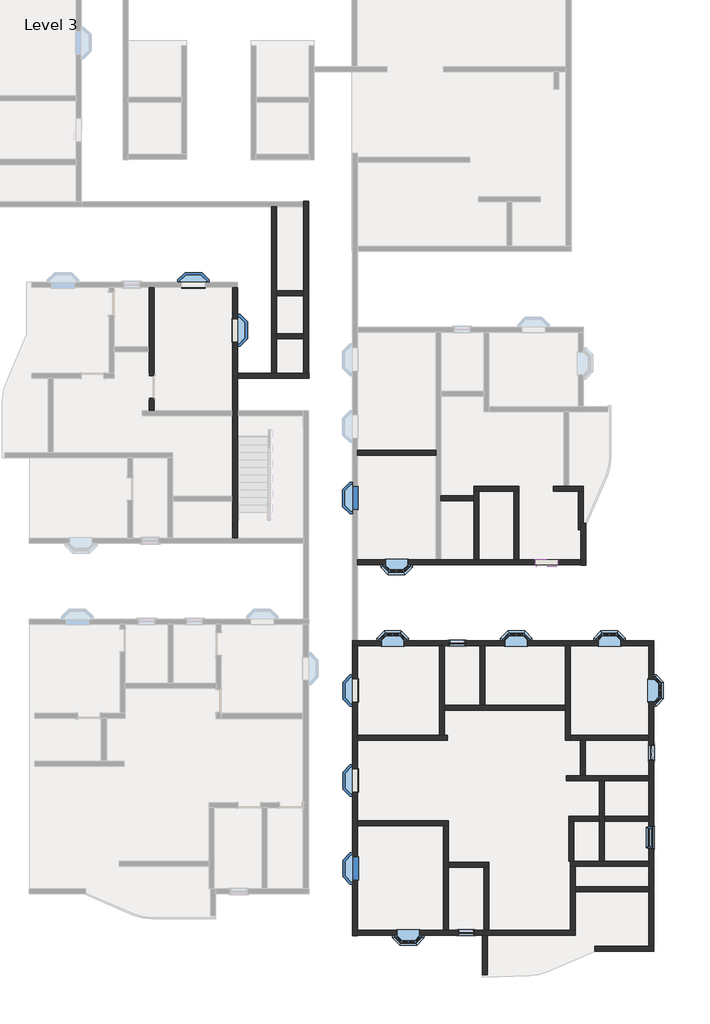
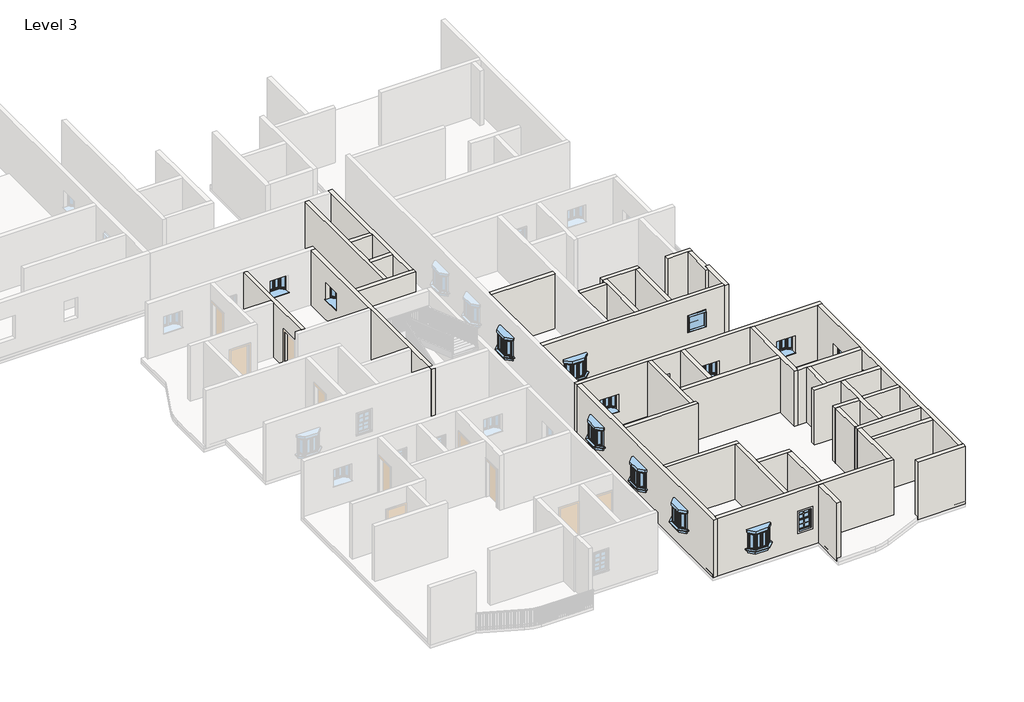
# One storey, part 2 of 14: 40 walls, 17 windows.
"""IFC4 building model written with IfcOpenShell, lengths in millimetres."""

from ifc_helpers import new_model, si_unit, frame, origin, place, context, project, spatial, polyline, outline, extrude, faceted_brep, transform, mapped, element, save
from components import window_910x910mm_67ef725a, window_8debb0fa, windows_sgl_w_glazing_bars_910x910mm_256712d0

model = new_model("IFC4")

# Units and contexts
model_context = context("Model", 3, world=origin())
ifc_project = project(units=[si_unit("LENGTHUNIT", "METRE", prefix="MILLI")], contexts=[model_context])

# Site, building, storey
site = spatial("IfcSite", under=ifc_project)
building = spatial("IfcBuilding", under=site)
storey = spatial("IfcBuildingStorey", under=building, Name="Level 3", Elevation=6096.0)

# Walls
placement = place(None, origin())
element("IfcWall", 1, ObjectType="4.5\" p", at=placement, inside=storey, context=model_context, shape_type="SweptSolid", body=[
    extrude(outline(polyline([(6070.4380523, -28382.7374148), (6070.4380523, -26796.6042694), (6273.6380523, -26796.6042694), (6273.6380523, -28382.7374148), (6070.4380523, -28382.7374148)])), frame((0.0, 0.0, 6096.0), z_axis=(0.0, 0.0, 1.0), x_axis=(1.0, 0.0, 0.0)), (0.0, 0.0, 1.0), 3048.0),
])
element("IfcWall", 2, ObjectType="4.5\" p", at=placement, inside=storey, context=model_context, shape_type="Brep", body=[
    faceted_brep([(10639.6896214, -27431.6042694, 6096.0), (13030.0380523, -27431.6042694, 6096.0), (13030.0380523, -27431.6042694, 9144.0), (10639.6896214, -27431.6042694, 9144.0), (10639.6896214, -27228.4042694, 6096.0), (10639.6896214, -27228.4042694, 9144.0), (12814.1380523, -27228.4042694, 9144.0), (13017.3380523, -27228.4042694, 9144.0), (13030.0380523, -27228.4042694, 9144.0), (13030.0380523, -27228.4042694, 6096.0), (13017.3380523, -27228.4042694, 6096.0), (12814.1380523, -27228.4042694, 6096.0)], [[[0, 1, 2, 3]], [[4, 5, 6, 7, 8, 9, 10, 11]], [[1, 0, 4, 11, 10, 9]], [[2, 1, 9, 8]], [[3, 2, 8, 7, 6, 5]], [[0, 3, 5, 4]]]),
])
element("IfcWall", 3, ObjectType="4.5\" p", at=placement, inside=storey, context=model_context, shape_type="Brep", body=[
    faceted_brep([(1015.8380523, -18878.1542694, 6096.0), (4648.0380523, -18878.1542694, 6096.0), (4648.0380523, -18878.1542694, 9144.0), (1015.8380523, -18878.1542694, 9144.0), (1015.8380523, -18674.9542694, 6096.0), (1015.8380523, -18674.9542694, 9144.0), (4336.8880523, -18674.9542694, 9144.0), (4540.0880523, -18674.9542694, 9144.0), (4648.0380523, -18674.9542694, 9144.0), (4648.0380523, -18674.9542694, 6096.0), (4540.0880523, -18674.9542694, 6096.0), (4336.8880523, -18674.9542694, 6096.0)], [[[0, 1, 2, 3]], [[4, 5, 6, 7, 8, 9, 10, 11]], [[1, 0, 4, 11, 10, 9]], [[2, 1, 9, 8]], [[3, 2, 8, 7, 6, 5]], [[0, 3, 5, 4]]]),
])
element("IfcWall", 4, ObjectType="4.5\" p", at=placement, inside=storey, context=model_context, shape_type="Brep", body=[
    faceted_brep([(4336.8880523, -15049.1042694, 6096.0), (4336.8880523, -18674.9542694, 6096.0), (4336.8880523, -18674.9542694, 9144.0), (4336.8880523, -15049.1042694, 9144.0), (4540.0880523, -15049.1042694, 6096.0), (4540.0880523, -15049.1042694, 9144.0), (4540.0880523, -17455.7542694, 9144.0), (4540.0880523, -17658.9542694, 9144.0), (4540.0880523, -18674.9542694, 9144.0), (4540.0880523, -18674.9542694, 6096.0), (4540.0880523, -17658.9542694, 6096.0), (4540.0880523, -17455.7542694, 6096.0)], [[[0, 1, 2, 3]], [[4, 5, 6, 7, 8, 9, 10, 11]], [[1, 0, 4, 11, 10, 9]], [[3, 2, 8, 7, 6, 5]], [[0, 3, 5, 4]], [[2, 1, 9, 8]]]),
])
element("IfcWall", 5, ObjectType="4.5\" p", at=placement, inside=storey, context=model_context, shape_type="Brep", body=[
    faceted_brep([(4540.0880523, -17658.9542694, 6096.0), (9442.2880523, -17658.9542694, 6096.0), (9442.2880523, -17658.9542694, 9144.0), (4540.0880523, -17658.9542694, 9144.0), (4540.0880523, -17455.7542694, 6096.0), (4540.0880523, -17455.7542694, 9144.0), (5975.1880523, -17455.7542694, 9144.0), (6178.3880523, -17455.7542694, 9144.0), (9442.2880523, -17455.7542694, 9144.0), (9442.2880523, -17455.7542694, 6096.0), (6178.3880523, -17455.7542694, 6096.0), (5975.1880523, -17455.7542694, 6096.0)], [[[0, 1, 2, 3]], [[4, 5, 6, 7, 8, 9, 10, 11]], [[1, 0, 4, 11, 10, 9]], [[3, 2, 8, 7, 6, 5]], [[0, 3, 5, 4]], [[2, 1, 9, 8]]]),
])
element("IfcWall", 6, ObjectType="4.5\" p", at=placement, inside=storey, context=model_context, shape_type="SweptSolid", body=[
    extrude(outline(polyline([(5975.1880523, -17455.7542694), (5975.1880523, -15049.1042694), (6178.3880523, -15049.1042694), (6178.3880523, -17455.7542694), (5975.1880523, -17455.7542694)])), frame((0.0, 0.0, 6096.0), z_axis=(0.0, 0.0, 1.0), x_axis=(1.0, 0.0, 0.0)), (0.0, 0.0, 1.0), 3048.0),
])
element("IfcWall", 7, ObjectType="4.5\" p", at=placement, inside=storey, context=model_context, shape_type="Brep", body=[
    faceted_brep([(9442.2880523, -15049.1042694, 6096.0), (9442.2880523, -17455.7542694, 6096.0), (9442.2880523, -17658.9542694, 6096.0), (9442.2880523, -18871.8042694, 6096.0), (9442.2880523, -18871.8042694, 9144.0), (9442.2880523, -17658.9542694, 9144.0), (9442.2880523, -17455.7542694, 9144.0), (9442.2880523, -15049.1042694, 9144.0), (9645.4880523, -15049.1042694, 6096.0), (9645.4880523, -15049.1042694, 9144.0), (9645.4880523, -18668.6042694, 9144.0), (9645.4880523, -18871.8042694, 9144.0), (9645.4880523, -18871.8042694, 6096.0), (9645.4880523, -18668.6042694, 6096.0)], [[[0, 1, 2, 3, 4, 5, 6, 7]], [[8, 9, 10, 11, 12, 13]], [[3, 2, 1, 0, 8, 13, 12]], [[7, 6, 5, 4, 11, 10, 9]], [[0, 7, 9, 8]], [[4, 3, 12, 11]]]),
])
element("IfcWall", 8, ObjectType="4.5\" p", at=placement, inside=storey, context=model_context, shape_type="Brep", body=[
    faceted_brep([(1015.8380523, -22345.2542694, 6096.0), (4489.2880523, -22345.2542694, 6096.0), (4692.4880523, -22345.2542694, 6096.0), (4692.4880523, -22345.2542694, 9144.0), (4489.2880523, -22345.2542694, 9144.0), (1015.8380523, -22345.2542694, 9144.0), (1015.8380523, -22142.0542694, 6096.0), (1015.8380523, -22142.0542694, 9144.0), (4692.4880523, -22142.0542694, 9144.0), (4692.4880523, -22142.0542694, 6096.0)], [[[0, 1, 2, 3, 4, 5]], [[6, 7, 8, 9]], [[2, 1, 0, 6, 9]], [[5, 4, 3, 8, 7]], [[0, 5, 7, 6]], [[3, 2, 9, 8]]]),
])
element("IfcWall", 9, ObjectType="4.5\" p", at=placement, inside=storey, context=model_context, shape_type="Brep", body=[
    faceted_brep([(4489.2880523, -22345.2542694, 6096.0), (4489.2880523, -26580.7042694, 6096.0), (4489.2880523, -26580.7042694, 9144.0), (4489.2880523, -22345.2542694, 9144.0), (4692.4880523, -22345.2542694, 6096.0), (4692.4880523, -22345.2542694, 9144.0), (4692.4880523, -23818.4542694, 9144.0), (4692.4880523, -24021.6542694, 9144.0), (4692.4880523, -26580.7042694, 9144.0), (4692.4880523, -26580.7042694, 6096.0), (4692.4880523, -24021.6542694, 6096.0), (4692.4880523, -23818.4542694, 6096.0)], [[[0, 1, 2, 3]], [[4, 5, 6, 7, 8, 9, 10, 11]], [[1, 0, 4, 11, 10, 9]], [[3, 2, 8, 7, 6, 5]], [[0, 3, 5, 4]], [[2, 1, 9, 8]]]),
])
element("IfcWall", 10, ObjectType="4.5\" p", at=placement, inside=storey, context=model_context, shape_type="Brep", body=[
    faceted_brep([(4692.4880523, -24021.6542694, 6096.0), (6127.5880523, -24021.6542694, 6096.0), (6330.7880523, -24021.6542694, 6096.0), (6330.7880523, -24021.6542694, 9144.0), (6127.5880523, -24021.6542694, 9144.0), (4692.4880523, -24021.6542694, 9144.0), (4692.4880523, -23818.4542694, 6096.0), (4692.4880523, -23818.4542694, 9144.0), (6330.7880523, -23818.4542694, 9144.0), (6330.7880523, -23818.4542694, 6096.0)], [[[0, 1, 2, 3, 4, 5]], [[6, 7, 8, 9]], [[2, 1, 0, 6, 9]], [[5, 4, 3, 8, 7]], [[0, 5, 7, 6]], [[3, 2, 9, 8]]]),
])
element("IfcWall", 11, ObjectType="4.5\" p", at=placement, inside=storey, context=model_context, shape_type="SweptSolid", body=[
    extrude(outline(polyline([(6127.5880523, -26580.7042694), (6127.5880523, -24021.6542694), (6330.7880523, -24021.6542694), (6330.7880523, -26580.7042694), (6127.5880523, -26580.7042694)])), frame((0.0, 0.0, 6096.0), z_axis=(0.0, 0.0, 1.0), x_axis=(1.0, 0.0, 0.0)), (0.0, 0.0, 1.0), 3048.0),
])
element("IfcWall", 12, ObjectType="4.5\" p", at=placement, inside=storey, context=model_context, shape_type="Brep", body=[
    faceted_brep([(9645.4880523, -18871.8042694, 6096.0), (10051.8880523, -18871.8042694, 6096.0), (10255.0880523, -18871.8042694, 6096.0), (12814.1380523, -18871.8042694, 6096.0), (12814.1380523, -18871.8042694, 9144.0), (10255.0880523, -18871.8042694, 9144.0), (10051.8880523, -18871.8042694, 9144.0), (9645.4880523, -18871.8042694, 9144.0), (9645.4880523, -18668.6042694, 6096.0), (9645.4880523, -18668.6042694, 9144.0), (12814.1380523, -18668.6042694, 9144.0), (12814.1380523, -18668.6042694, 6096.0)], [[[0, 1, 2, 3, 4, 5, 6, 7]], [[8, 9, 10, 11]], [[3, 2, 1, 0, 8, 11]], [[7, 6, 5, 4, 10, 9]], [[0, 7, 9, 8]], [[4, 3, 11, 10]]]),
])
element("IfcWall", 13, ObjectType="4.5\" p", at=placement, inside=storey, context=model_context, shape_type="SweptSolid", body=[
    extrude(outline(polyline([(10051.8880523, -20313.2542694), (10051.8880523, -18871.8042694), (10255.0880523, -18871.8042694), (10255.0880523, -20313.2542694), (10051.8880523, -20313.2542694)])), frame((0.0, 0.0, 6096.0), z_axis=(0.0, 0.0, 1.0), x_axis=(1.0, 0.0, 0.0)), (0.0, 0.0, 1.0), 3048.0),
])
element("IfcWall", 14, ObjectType="4.5\" p", at=placement, inside=storey, context=model_context, shape_type="Brep", body=[
    faceted_brep([(12814.1380523, -20313.2542694, 6096.0), (10255.0880523, -20313.2542694, 6096.0), (10051.8880523, -20313.2542694, 6096.0), (9486.7380523, -20313.2542694, 6096.0), (9486.7380523, -20313.2542694, 9144.0), (10051.8880523, -20313.2542694, 9144.0), (10255.0880523, -20313.2542694, 9144.0), (12814.1380523, -20313.2542694, 9144.0), (12814.1380523, -20516.4542694, 6096.0), (12814.1380523, -20516.4542694, 9144.0), (11017.0880523, -20516.4542694, 9144.0), (10813.8880523, -20516.4542694, 9144.0), (9486.7380523, -20516.4542694, 9144.0), (9486.7380523, -20516.4542694, 6096.0), (10813.8880523, -20516.4542694, 6096.0), (11017.0880523, -20516.4542694, 6096.0)], [[[0, 1, 2, 3, 4, 5, 6, 7]], [[8, 9, 10, 11, 12, 13, 14, 15]], [[3, 2, 1, 0, 8, 15, 14, 13]], [[4, 3, 13, 12]], [[7, 6, 5, 4, 12, 11, 10, 9]], [[0, 7, 9, 8]]]),
])
element("IfcWall", 15, ObjectType="4.5\" p", at=placement, inside=storey, context=model_context, shape_type="Brep", body=[
    faceted_brep([(10813.8880523, -20516.4542694, 6096.0), (10813.8880523, -21951.5542694, 6096.0), (10813.8880523, -22154.7542694, 6096.0), (10813.8880523, -23779.5416506, 6096.0), (10813.8880523, -23779.5416506, 9144.0), (10813.8880523, -22154.7542694, 9144.0), (10813.8880523, -21951.5542694, 9144.0), (10813.8880523, -20516.4542694, 9144.0), (11017.0880523, -20516.4542694, 6096.0), (11017.0880523, -20516.4542694, 9144.0), (11017.0880523, -21951.5542694, 9144.0), (11017.0880523, -22154.7542694, 9144.0), (11017.0880523, -23779.5416506, 9144.0), (11017.0880523, -23779.5416506, 6096.0), (11017.0880523, -22154.7542694, 6096.0), (11017.0880523, -21951.5542694, 6096.0)], [[[0, 1, 2, 3, 4, 5, 6, 7]], [[8, 9, 10, 11, 12, 13, 14, 15]], [[3, 2, 1, 0, 8, 15, 14, 13]], [[7, 6, 5, 4, 12, 11, 10, 9]], [[0, 7, 9, 8]], [[4, 3, 13, 12]]]),
])
element("IfcWall", 16, ObjectType="4.5\" p", at=placement, inside=storey, context=model_context, shape_type="Brep", body=[
    faceted_brep([(12814.1380523, -23779.5416506, 6096.0), (11017.0880523, -23779.5416506, 6096.0), (10813.8880523, -23779.5416506, 6096.0), (9791.5380523, -23779.5416506, 6096.0), (9632.7880523, -23779.5416506, 6096.0), (9632.7880523, -23779.5416506, 9144.0), (9791.5380523, -23779.5416506, 9144.0), (10813.8880523, -23779.5416506, 9144.0), (11017.0880523, -23779.5416506, 9144.0), (12814.1380523, -23779.5416506, 9144.0), (12814.1380523, -23982.7416506, 6096.0), (12814.1380523, -23982.7416506, 9144.0), (9835.9880523, -23982.7416506, 9144.0), (9632.7880523, -23982.7416506, 9144.0), (9632.7880523, -23982.7416506, 6096.0), (9835.9880523, -23982.7416506, 6096.0)], [[[0, 1, 2, 3, 4, 5, 6, 7, 8, 9]], [[10, 11, 12, 13, 14, 15]], [[4, 3, 2, 1, 0, 10, 15, 14]], [[9, 8, 7, 6, 5, 13, 12, 11]], [[0, 9, 11, 10]], [[5, 4, 14, 13]]]),
])
element("IfcWall", 17, ObjectType="4.5\" p", at=placement, inside=storey, context=model_context, shape_type="Brep", body=[
    faceted_brep([(9632.7880523, -23982.7416506, 6096.0), (9632.7880523, -26580.7042694, 6096.0), (9632.7880523, -26580.7042694, 9144.0), (9632.7880523, -23982.7416506, 9144.0), (9835.9880523, -23982.7416506, 6096.0), (9835.9880523, -23982.7416506, 9144.0), (9835.9880523, -24805.3496998, 9144.0), (9835.9880523, -25008.5496998, 9144.0), (9835.9880523, -26580.7042694, 9144.0), (9835.9880523, -26580.7042694, 6096.0), (9835.9880523, -25008.5496998, 6096.0), (9835.9880523, -24805.3496998, 6096.0)], [[[0, 1, 2, 3]], [[4, 5, 6, 7, 8, 9, 10, 11]], [[1, 0, 4, 11, 10, 9]], [[3, 2, 8, 7, 6, 5]], [[2, 1, 9, 8]], [[0, 3, 5, 4]]]),
])
element("IfcWall", 18, ObjectType="4.5\" p", at=placement, inside=storey, context=model_context, shape_type="SweptSolid", body=[
    extrude(outline(polyline([(12814.1380523, -25008.5496998), (9835.9880523, -25008.5496998), (9835.9880523, -24805.3496998), (12814.1380523, -24805.3496998), (12814.1380523, -25008.5496998)])), frame((0.0, 0.0, 6096.0), z_axis=(0.0, 0.0, 1.0), x_axis=(1.0, 0.0, 0.0)), (0.0, 0.0, 1.0), 3048.0),
])
element("IfcWall", 19, ObjectType="4.5\" p", at=placement, inside=storey, context=model_context, shape_type="Brep", body=[
    faceted_brep([(-7432.737215, -5015.2916506, 8229.6), (-7432.737215, -5015.2916506, 6096.0), (-7432.737215, -5523.2916506, 6096.0), (-7432.737215, -5523.2916506, 9144.0), (-7432.737215, -3135.6916506, 9144.0), (-7432.737215, -2932.4916506, 9144.0), (-7432.737215, -525.8416506, 9144.0), (-7432.737215, -525.8416506, 6096.0), (-7432.737215, -2932.4916506, 6096.0), (-7432.737215, -3135.6916506, 6096.0), (-7432.737215, -4100.8916506, 6096.0), (-7432.737215, -4100.8916506, 8229.6), (-7229.537215, -5523.2916506, 6096.0), (-7229.537215, -5015.2916506, 6096.0), (-7229.537215, -5015.2916506, 8229.6), (-7229.537215, -4100.8916506, 8229.6), (-7229.537215, -4100.8916506, 6096.0), (-7229.537215, -525.8416506, 6096.0), (-7229.537215, -525.8416506, 9144.0), (-7229.537215, -5523.2916506, 9144.0)], [[[0, 1, 2, 3, 4, 5, 6, 7, 8, 9, 10, 11]], [[12, 13, 14, 15, 16, 17, 18, 19]], [[2, 1, 13, 12]], [[10, 9, 8, 7, 17, 16]], [[6, 5, 4, 3, 19, 18]], [[7, 6, 18, 17]], [[3, 2, 12, 19]], [[14, 13, 1, 0]], [[15, 14, 0, 11]], [[16, 15, 11, 10]]]),
])
element("IfcWall", 20, ObjectType="4.5\" p", at=placement, inside=storey, context=model_context, shape_type="Brep", body=[
    faceted_brep([(-3857.687215, -4202.4916506, 6096.0), (-961.4891351, -4202.4916506, 6096.0), (-961.4891351, -4202.4916506, 9144.0), (-3857.687215, -4202.4916506, 9144.0), (-3857.687215, -3999.2916506, 6096.0), (-3857.687215, -3999.2916506, 9144.0), (-2472.7891351, -3999.2916506, 9144.0), (-2269.5891351, -3999.2916506, 9144.0), (-1177.3891351, -3999.2916506, 9144.0), (-974.1891351, -3999.2916506, 9144.0), (-961.4891351, -3999.2916506, 9144.0), (-961.4891351, -3999.2916506, 6096.0), (-974.1891351, -3999.2916506, 6096.0), (-1177.3891351, -3999.2916506, 6096.0), (-2269.5891351, -3999.2916506, 6096.0), (-2472.7891351, -3999.2916506, 6096.0)], [[[0, 1, 2, 3]], [[4, 5, 6, 7, 8, 9, 10, 11, 12, 13, 14, 15]], [[1, 0, 4, 15, 14, 13, 12, 11]], [[2, 1, 11, 10]], [[3, 2, 10, 9, 8, 7, 6, 5]], [[0, 3, 5, 4]]]),
])
element("IfcWall", 21, ObjectType="4.5\" p", at=placement, inside=storey, context=model_context, shape_type="SweptSolid", body=[
    extrude(outline(polyline([(-1177.3891351, -868.7416506), (-2269.5891351, -868.7416506), (-2269.5891351, -665.5416506), (-1177.3891351, -665.5416506), (-1177.3891351, -868.7416506)])), frame((0.0, 0.0, 6096.0), z_axis=(0.0, 0.0, 1.0), x_axis=(1.0, 0.0, 0.0)), (0.0, 0.0, 1.0), 3048.0),
])
element("IfcWall", 22, ObjectType="4.5\" p", at=placement, inside=storey, context=model_context, shape_type="SweptSolid", body=[
    extrude(outline(polyline([(-1177.3891351, -2597.8466506), (-2269.5891351, -2597.8466506), (-2269.5891351, -2394.6466506), (-1177.3891351, -2394.6466506), (-1177.3891351, -2597.8466506)])), frame((0.0, 0.0, 6096.0), z_axis=(0.0, 0.0, 1.0), x_axis=(1.0, 0.0, 0.0)), (0.0, 0.0, 1.0), 3048.0),
])
element("IfcWall", 23, ObjectType="4.5\" p", at=placement, inside=storey, context=model_context, shape_type="SweptSolid", body=[
    extrude(outline(polyline([(5721.1880523, -9162.6542694), (4387.6880523, -9162.6542694), (4387.6880523, -8959.4542694), (5721.1880523, -8959.4542694), (5721.1880523, -9162.6542694)])), frame((0.0, 0.0, 6096.0), z_axis=(0.0, 0.0, 1.0), x_axis=(1.0, 0.0, 0.0)), (0.0, 0.0, 1.0), 3048.0),
])
element("IfcWall", 24, ObjectType="4.5\" p", at=placement, inside=storey, context=model_context, shape_type="Brep", body=[
    faceted_brep([(5721.1880523, -8781.6542694, 6096.0), (5924.3880523, -8781.6542694, 6096.0), (7359.4880523, -8781.6542694, 6096.0), (7562.6880523, -8781.6542694, 6096.0), (7562.6880523, -8781.6542694, 9144.0), (7359.4880523, -8781.6542694, 9144.0), (5924.3880523, -8781.6542694, 9144.0), (5721.1880523, -8781.6542694, 9144.0), (5721.1880523, -8578.4542694, 6096.0), (5721.1880523, -8578.4542694, 9144.0), (7562.6880523, -8578.4542694, 9144.0), (7562.6880523, -8578.4542694, 6096.0)], [[[0, 1, 2, 3, 4, 5, 6, 7]], [[8, 9, 10, 11]], [[3, 2, 1, 0, 8, 11]], [[7, 6, 5, 4, 10, 9]], [[0, 7, 9, 8]], [[4, 3, 11, 10]]]),
])
element("IfcWall", 25, ObjectType="4.5\" p", at=placement, inside=storey, context=model_context, shape_type="Brep", body=[
    faceted_brep([(5721.1880523, -8781.6542694, 6096.0), (5721.1880523, -8959.4542694, 6096.0), (5721.1880523, -9162.6542694, 6096.0), (5721.1880523, -11556.6042694, 6096.0), (5721.1880523, -11556.6042694, 9144.0), (5721.1880523, -9162.6542694, 9144.0), (5721.1880523, -8959.4542694, 9144.0), (5721.1880523, -8781.6542694, 9144.0), (5924.3880523, -8781.6542694, 6096.0), (5924.3880523, -8781.6542694, 9144.0), (5924.3880523, -11556.6042694, 9144.0), (5924.3880523, -11556.6042694, 6096.0)], [[[0, 1, 2, 3, 4, 5, 6, 7]], [[8, 9, 10, 11]], [[3, 2, 1, 0, 8, 11]], [[7, 6, 5, 4, 10, 9]], [[0, 7, 9, 8]], [[4, 3, 11, 10]]]),
])
element("IfcWall", 26, ObjectType="4.5\" p", at=placement, inside=storey, context=model_context, shape_type="SweptSolid", body=[
    extrude(outline(polyline([(7359.4880523, -11556.6042694), (7359.4880523, -8781.6542694), (7562.6880523, -8781.6542694), (7562.6880523, -11556.6042694), (7359.4880523, -11556.6042694)])), frame((0.0, 0.0, 6096.0), z_axis=(0.0, 0.0, 1.0), x_axis=(1.0, 0.0, 0.0)), (0.0, 0.0, 1.0), 3048.0),
])
element("IfcWall", 27, ObjectType="4.5\" p", at=placement, inside=storey, context=model_context, shape_type="SweptSolid", body=[
    extrude(outline(polyline([(4184.4880523, -7333.8542694), (1007.0108649, -7333.8542694), (1007.0108649, -7130.6542694), (4184.4880523, -7130.6542694), (4184.4880523, -7333.8542694)])), frame((0.0, 0.0, 6096.0), z_axis=(0.0, 0.0, 1.0), x_axis=(1.0, 0.0, 0.0)), (0.0, 0.0, 1.0), 3048.0),
])
element("IfcWall", 28, ObjectType="4.5\" p", at=placement, inside=storey, context=model_context, shape_type="Brep", body=[
    faceted_brep([(8953.3380523, -8781.6542694, 6096.0), (9956.6380523, -8781.6542694, 6096.0), (10159.8380523, -8781.6542694, 6096.0), (10172.5380523, -8781.6542694, 6096.0), (10172.5380523, -8781.6542694, 9144.0), (10159.8380523, -8781.6542694, 9144.0), (9956.6380523, -8781.6542694, 9144.0), (8953.3380523, -8781.6542694, 9144.0), (8953.3380523, -8578.4542694, 6096.0), (8953.3380523, -8578.4542694, 9144.0), (9371.2322031, -8578.4542694, 9144.0), (9574.4322031, -8578.4542694, 9144.0), (10172.5380523, -8578.4542694, 9144.0), (10172.5380523, -8578.4542694, 6096.0), (9574.4322031, -8578.4542694, 6096.0), (9371.2322031, -8578.4542694, 6096.0)], [[[0, 1, 2, 3, 4, 5, 6, 7]], [[8, 9, 10, 11, 12, 13, 14, 15]], [[3, 2, 1, 0, 8, 15, 14, 13]], [[4, 3, 13, 12]], [[7, 6, 5, 4, 12, 11, 10, 9]], [[0, 7, 9, 8]]]),
])
element("IfcWall", 29, ObjectType="4.5\" p", at=placement, inside=storey, context=model_context, shape_type="SweptSolid", body=[
    extrude(outline(polyline([(9956.6380523, -10352.8912671), (9956.6380523, -8781.6542694), (10159.8380523, -8781.6542694), (10159.8380523, -10352.8912671), (9956.6380523, -10352.8912671)])), frame((0.0, 0.0, 6096.0), z_axis=(0.0, 0.0, 1.0), x_axis=(1.0, 0.0, 0.0)), (0.0, 0.0, 1.0), 3048.0),
])
element("IfcWall", 30, ObjectType="4.5\" p", at=placement, inside=storey, context=model_context, shape_type="Brep", body=[
    faceted_brep([(12814.1380523, -21951.5542694, 9144.0), (12814.1380523, -21951.5542694, 6096.0), (11017.0880523, -21951.5542694, 6096.0), (11017.0880523, -21951.5542694, 9144.0), (12814.1380523, -22154.7542694, 6096.0), (12814.1380523, -22154.7542694, 9144.0), (11017.0880523, -22154.7542694, 9144.0), (11017.0880523, -22154.7542694, 6096.0)], [[[0, 1, 2, 3]], [[4, 5, 6, 7]], [[1, 4, 7, 2]], [[5, 0, 3, 6]], [[1, 0, 5, 4]], [[3, 2, 7, 6]]]),
    faceted_brep([(9588.3380523, -21951.5542694, 6096.0), (9588.3380523, -21951.5542694, 9144.0), (10813.8880523, -21951.5542694, 9144.0), (10813.8880523, -21951.5542694, 6096.0), (9588.3380523, -22154.7542694, 9144.0), (9588.3380523, -22154.7542694, 6096.0), (9791.5380523, -22154.7542694, 6096.0), (10813.8880523, -22154.7542694, 6096.0), (10813.8880523, -22154.7542694, 9144.0), (9791.5380523, -22154.7542694, 9144.0)], [[[0, 1, 2, 3]], [[4, 5, 6, 7, 8, 9]], [[5, 0, 3, 7, 6]], [[1, 4, 9, 8, 2]], [[3, 2, 8, 7]], [[1, 0, 5, 4]]]),
])
element("IfcWall", 31, ObjectType="4.5\" p", at=placement, inside=storey, context=model_context, shape_type="Brep", body=[
    faceted_brep([(9588.3380523, -22154.7542694, 6096.0), (9588.3380523, -23779.5416506, 6096.0), (9588.3380523, -23779.5416506, 9144.0), (9588.3380523, -22154.7542694, 9144.0), (9791.5380523, -22154.7542694, 6096.0), (9791.5380523, -22154.7542694, 9144.0), (9791.5380523, -23779.5416506, 9144.0), (9791.5380523, -23779.5416506, 6096.0), (9632.7880523, -23779.5416506, 6096.0), (9632.7880523, -23779.5416506, 9144.0)], [[[0, 1, 2, 3]], [[4, 5, 6, 7]], [[1, 0, 4, 7, 8]], [[3, 2, 9, 6, 5]], [[2, 1, 8, 7, 6, 9]], [[0, 3, 5, 4]]]),
])
element("IfcWall", 32, ObjectType="9\"", at=placement, inside=storey, context=model_context, shape_type="Brep", body=[
    faceted_brep([(799.9380523, -15049.1042694, 6096.0), (812.6380523, -15049.1042694, 6096.0), (1015.8380523, -15049.1042694, 6096.0), (4336.8880523, -15049.1042694, 6096.0), (4540.0880523, -15049.1042694, 6096.0), (5975.1880523, -15049.1042694, 6096.0), (6178.3880523, -15049.1042694, 6096.0), (9442.2880523, -15049.1042694, 6096.0), (9645.4880523, -15049.1042694, 6096.0), (12814.1380523, -15049.1042694, 6096.0), (13017.3380523, -15049.1042694, 6096.0), (13030.0380523, -15049.1042694, 6096.0), (13030.0380523, -15049.1042694, 9144.0), (13017.3380523, -15049.1042694, 9144.0), (12814.1380523, -15049.1042694, 9144.0), (9645.4880523, -15049.1042694, 9144.0), (9442.2880523, -15049.1042694, 9144.0), (6178.3880523, -15049.1042694, 9144.0), (5975.1880523, -15049.1042694, 9144.0), (4540.0880523, -15049.1042694, 9144.0), (4336.8880523, -15049.1042694, 9144.0), (1015.8380523, -15049.1042694, 9144.0), (812.6380523, -15049.1042694, 9144.0), (799.9380523, -15049.1042694, 9144.0), (1983.2380523, -15049.1042694, 7920.4), (2893.2380523, -15049.1042694, 7920.4), (2893.2380523, -15049.1042694, 7010.4), (1983.2380523, -15049.1042694, 7010.4), (10774.8130523, -15049.1042694, 7920.4), (11684.8130523, -15049.1042694, 7920.4), (11684.8130523, -15049.1042694, 7010.4), (10774.8130523, -15049.1042694, 7010.4), (6993.3880523, -15049.1042694, 7920.4), (7903.3880523, -15049.1042694, 7920.4), (7903.3880523, -15049.1042694, 7010.4), (6993.3880523, -15049.1042694, 7010.4), (4717.8880523, -15049.1042694, 8077.2), (5378.2880523, -15049.1042694, 8077.2), (5378.2880523, -15049.1042694, 7010.4), (4717.8880523, -15049.1042694, 7010.4), (799.9380523, -14845.9042694, 6096.0), (799.9380523, -14845.9042694, 9144.0), (803.8108649, -14845.9042694, 9144.0), (1007.0108649, -14845.9042694, 9144.0), (13030.0380523, -14845.9042694, 9144.0), (13030.0380523, -14845.9042694, 6096.0), (1007.0108649, -14845.9042694, 6096.0), (803.8108649, -14845.9042694, 6096.0), (1983.2380523, -14845.9042694, 7920.4), (1983.2380523, -14845.9042694, 7010.4), (2893.2380523, -14845.9042694, 7010.4), (2893.2380523, -14845.9042694, 7920.4), (10774.8130523, -14845.9042694, 7920.4), (10774.8130523, -14845.9042694, 7010.4), (11684.8130523, -14845.9042694, 7010.4), (11684.8130523, -14845.9042694, 7920.4), (6993.3880523, -14845.9042694, 7920.4), (6993.3880523, -14845.9042694, 7010.4), (7903.3880523, -14845.9042694, 7010.4), (7903.3880523, -14845.9042694, 7920.4), (4717.8880523, -14845.9042694, 8077.2), (4717.8880523, -14845.9042694, 7010.4), (5378.2880523, -14845.9042694, 7010.4), (5378.2880523, -14845.9042694, 8077.2)], [[[0, 1, 2, 3, 4, 5, 6, 7, 8, 9, 10, 11, 12, 13, 14, 15, 16, 17, 18, 19, 20, 21, 22, 23], [24, 25, 26, 27], [28, 29, 30, 31], [32, 33, 34, 35], [36, 37, 38, 39]], [[40, 41, 42, 43, 44, 45, 46, 47], [48, 49, 50, 51], [52, 53, 54, 55], [56, 57, 58, 59], [60, 61, 62, 63]], [[11, 10, 9, 8, 7, 6, 5, 4, 3, 2, 1, 0, 40, 47, 46, 45]], [[12, 11, 45, 44]], [[23, 22, 21, 20, 19, 18, 17, 16, 15, 14, 13, 12, 44, 43, 42, 41]], [[0, 23, 41, 40]], [[49, 48, 24, 27]], [[50, 49, 27, 26]], [[51, 50, 26, 25]], [[48, 51, 25, 24]], [[53, 52, 28, 31]], [[54, 53, 31, 30]], [[55, 54, 30, 29]], [[52, 55, 29, 28]], [[57, 56, 32, 35]], [[58, 57, 35, 34]], [[59, 58, 34, 33]], [[56, 59, 33, 32]], [[61, 60, 36, 39]], [[62, 61, 39, 38]], [[63, 62, 38, 37]], [[60, 63, 37, 36]]]),
])
element("IfcWall", 33, ObjectType="9\"", at=placement, inside=storey, context=model_context, shape_type="Brep", body=[
    faceted_brep([(12814.1380523, -15049.1042694, 6096.0), (12814.1380523, -18668.6042694, 6096.0), (12814.1380523, -18871.8042694, 6096.0), (12814.1380523, -20313.2542694, 6096.0), (12814.1380523, -20516.4542694, 6096.0), (12814.1380523, -21951.5542694, 6096.0), (12814.1380523, -22154.7542694, 6096.0), (12814.1380523, -23779.5416506, 6096.0), (12814.1380523, -23982.7416506, 6096.0), (12814.1380523, -24805.3496998, 6096.0), (12814.1380523, -25008.5496998, 6096.0), (12814.1380523, -27228.4042694, 6096.0), (12814.1380523, -27228.4042694, 9144.0), (12814.1380523, -25008.5496998, 9144.0), (12814.1380523, -24805.3496998, 9144.0), (12814.1380523, -23982.7416506, 9144.0), (12814.1380523, -23779.5416506, 9144.0), (12814.1380523, -22154.7542694, 9144.0), (12814.1380523, -21951.5542694, 9144.0), (12814.1380523, -20516.4542694, 9144.0), (12814.1380523, -20313.2542694, 9144.0), (12814.1380523, -18871.8042694, 9144.0), (12814.1380523, -18668.6042694, 9144.0), (12814.1380523, -15049.1042694, 9144.0), (12814.1380523, -16403.8542694, 7920.4), (12814.1380523, -17313.8542694, 7920.4), (12814.1380523, -17313.8542694, 7010.4), (12814.1380523, -16403.8542694, 7010.4), (12814.1380523, -23270.1542694, 7920.4), (12814.1380523, -23270.1542694, 7010.4), (12814.1380523, -22360.1542694, 7010.4), (12814.1380523, -22360.1542694, 7920.4), (12814.1380523, -19049.6042694, 8077.2), (12814.1380523, -19710.0042694, 8077.2), (12814.1380523, -19710.0042694, 7010.4), (12814.1380523, -19049.6042694, 7010.4), (13017.3380523, -15049.1042694, 6096.0), (13017.3380523, -15049.1042694, 9144.0), (13017.3380523, -27228.4042694, 9144.0), (13017.3380523, -27228.4042694, 6096.0), (13017.3380523, -16403.8542694, 7920.4), (13017.3380523, -16403.8542694, 7010.4), (13017.3380523, -17313.8542694, 7010.4), (13017.3380523, -17313.8542694, 7920.4), (13017.3380523, -23270.1542694, 7920.4), (13017.3380523, -22360.1542694, 7920.4), (13017.3380523, -22360.1542694, 7010.4), (13017.3380523, -23270.1542694, 7010.4), (13017.3380523, -19049.6042694, 8077.2), (13017.3380523, -19049.6042694, 7010.4), (13017.3380523, -19710.0042694, 7010.4), (13017.3380523, -19710.0042694, 8077.2)], [[[0, 1, 2, 3, 4, 5, 6, 7, 8, 9, 10, 11, 12, 13, 14, 15, 16, 17, 18, 19, 20, 21, 22, 23], [24, 25, 26, 27], [28, 29, 30, 31], [32, 33, 34, 35]], [[36, 37, 38, 39], [40, 41, 42, 43], [44, 45, 46, 47], [48, 49, 50, 51]], [[11, 10, 9, 8, 7, 6, 5, 4, 3, 2, 1, 0, 36, 39]], [[23, 22, 21, 20, 19, 18, 17, 16, 15, 14, 13, 12, 38, 37]], [[0, 23, 37, 36]], [[12, 11, 39, 38]], [[41, 40, 24, 27]], [[42, 41, 27, 26]], [[43, 42, 26, 25]], [[40, 43, 25, 24]], [[29, 28, 44, 47]], [[30, 29, 47, 46]], [[31, 30, 46, 45]], [[28, 31, 45, 44]], [[49, 48, 32, 35]], [[50, 49, 35, 34]], [[51, 50, 34, 33]], [[48, 51, 33, 32]]]),
])
element("IfcWall", 34, ObjectType="9\"", at=placement, inside=storey, context=model_context, shape_type="Brep", body=[
    faceted_brep([(812.6380523, -15049.1042694, 6096.0), (812.6380523, -26796.6042694, 6096.0), (812.6380523, -26796.6042694, 9144.0), (812.6380523, -15049.1042694, 9144.0), (812.6380523, -24527.4542694, 8206.0), (812.6380523, -24527.4542694, 7296.0), (812.6380523, -23617.4542694, 7296.0), (812.6380523, -23617.4542694, 8206.0), (812.6380523, -20965.1042694, 8206.0), (812.6380523, -20965.1042694, 7296.0), (812.6380523, -20055.1042694, 7296.0), (812.6380523, -20055.1042694, 8206.0), (812.6380523, -17317.0292694, 8206.0), (812.6380523, -17317.0292694, 7296.0), (812.6380523, -16407.0292694, 7296.0), (812.6380523, -16407.0292694, 8206.0), (1015.8380523, -15049.1042694, 6096.0), (1015.8380523, -15049.1042694, 9144.0), (1015.8380523, -18674.9542694, 9144.0), (1015.8380523, -18878.1542694, 9144.0), (1015.8380523, -22142.0542694, 9144.0), (1015.8380523, -22345.2542694, 9144.0), (1015.8380523, -26580.7042694, 9144.0), (1015.8380523, -26783.9042694, 9144.0), (1015.8380523, -26796.6042694, 9144.0), (1015.8380523, -26796.6042694, 6096.0), (1015.8380523, -26783.9042694, 6096.0), (1015.8380523, -26580.7042694, 6096.0), (1015.8380523, -22345.2542694, 6096.0), (1015.8380523, -22142.0542694, 6096.0), (1015.8380523, -18878.1542694, 6096.0), (1015.8380523, -18674.9542694, 6096.0), (1015.8380523, -24527.4542694, 8206.0), (1015.8380523, -23617.4542694, 8206.0), (1015.8380523, -23617.4542694, 7296.0), (1015.8380523, -24527.4542694, 7296.0), (1015.8380523, -20965.1042694, 8206.0), (1015.8380523, -20055.1042694, 8206.0), (1015.8380523, -20055.1042694, 7296.0), (1015.8380523, -20965.1042694, 7296.0), (1015.8380523, -17317.0292694, 8206.0), (1015.8380523, -16407.0292694, 8206.0), (1015.8380523, -16407.0292694, 7296.0), (1015.8380523, -17317.0292694, 7296.0)], [[[0, 1, 2, 3], [4, 5, 6, 7], [8, 9, 10, 11], [12, 13, 14, 15]], [[16, 17, 18, 19, 20, 21, 22, 23, 24, 25, 26, 27, 28, 29, 30, 31], [32, 33, 34, 35], [36, 37, 38, 39], [40, 41, 42, 43]], [[1, 0, 16, 31, 30, 29, 28, 27, 26, 25]], [[2, 1, 25, 24]], [[3, 2, 24, 23, 22, 21, 20, 19, 18, 17]], [[0, 3, 17, 16]], [[5, 4, 32, 35]], [[6, 5, 35, 34]], [[7, 6, 34, 33]], [[4, 7, 33, 32]], [[9, 8, 36, 39]], [[10, 9, 39, 38]], [[11, 10, 38, 37]], [[8, 11, 37, 36]], [[13, 12, 40, 43]], [[14, 13, 43, 42]], [[15, 14, 42, 41]], [[12, 15, 41, 40]]]),
])
element("IfcWall", 35, ObjectType="9\"", at=placement, inside=storey, context=model_context, shape_type="Brep", body=[
    faceted_brep([(1015.8380523, -26783.9042694, 6096.0), (9835.9880523, -26783.9042694, 6096.0), (9835.9880523, -26783.9042694, 9144.0), (1015.8380523, -26783.9042694, 9144.0), (3521.8880523, -26783.9042694, 7920.4), (3521.8880523, -26783.9042694, 7010.4), (2611.8880523, -26783.9042694, 7010.4), (2611.8880523, -26783.9042694, 7920.4), (5079.8380523, -26783.9042694, 8077.2), (5740.2380523, -26783.9042694, 8077.2), (5740.2380523, -26783.9042694, 7010.4), (5079.8380523, -26783.9042694, 7010.4), (1015.8380523, -26580.7042694, 6096.0), (1015.8380523, -26580.7042694, 9144.0), (4489.2880523, -26580.7042694, 9144.0), (4692.4880523, -26580.7042694, 9144.0), (6127.5880523, -26580.7042694, 9144.0), (6330.7880523, -26580.7042694, 9144.0), (9632.7880523, -26580.7042694, 9144.0), (9835.9880523, -26580.7042694, 9144.0), (9835.9880523, -26580.7042694, 6096.0), (9632.7880523, -26580.7042694, 6096.0), (6330.7880523, -26580.7042694, 6096.0), (6127.5880523, -26580.7042694, 6096.0), (4692.4880523, -26580.7042694, 6096.0), (4489.2880523, -26580.7042694, 6096.0), (3521.8880523, -26580.7042694, 7920.4), (2611.8880523, -26580.7042694, 7920.4), (2611.8880523, -26580.7042694, 7010.4), (3521.8880523, -26580.7042694, 7010.4), (5079.8380523, -26580.7042694, 8077.2), (5079.8380523, -26580.7042694, 7010.4), (5740.2380523, -26580.7042694, 7010.4), (5740.2380523, -26580.7042694, 8077.2)], [[[0, 1, 2, 3], [4, 5, 6, 7], [8, 9, 10, 11]], [[12, 13, 14, 15, 16, 17, 18, 19, 20, 21, 22, 23, 24, 25], [26, 27, 28, 29], [30, 31, 32, 33]], [[1, 0, 12, 25, 24, 23, 22, 21, 20]], [[3, 2, 19, 18, 17, 16, 15, 14, 13]], [[0, 3, 13, 12]], [[2, 1, 20, 19]], [[5, 4, 26, 29]], [[6, 5, 29, 28]], [[7, 6, 28, 27]], [[4, 7, 27, 26]], [[31, 30, 8, 11]], [[32, 31, 11, 10]], [[33, 32, 10, 9]], [[30, 33, 9, 8]]]),
])
element("IfcWall", 36, ObjectType="9\" w", at=placement, inside=storey, context=model_context, shape_type="Brep", body=[
    faceted_brep([(-4060.887215, -525.8416506, 6096.0), (-4060.887215, -5523.2916506, 6096.0), (-4060.887215, -5726.4916506, 6096.0), (-4060.887215, -8990.3916506, 6096.0), (-4060.887215, -9193.5916506, 6096.0), (-4060.887215, -10901.7416506, 6096.0), (-4060.887215, -10901.7416506, 9144.0), (-4060.887215, -9193.5916506, 9144.0), (-4060.887215, -8990.3916506, 9144.0), (-4060.887215, -5726.4916506, 9144.0), (-4060.887215, -5523.2916506, 9144.0), (-4060.887215, -525.8416506, 9144.0), (-4060.887215, -1807.5666506, 8206.0), (-4060.887215, -2717.5666506, 8206.0), (-4060.887215, -2717.5666506, 7296.0), (-4060.887215, -1807.5666506, 7296.0), (-3857.687215, -525.8416506, 6096.0), (-3857.687215, -525.8416506, 9144.0), (-3857.687215, -3999.2916506, 9144.0), (-3857.687215, -4202.4916506, 9144.0), (-3857.687215, -5523.2916506, 9144.0), (-3857.687215, -5726.4916506, 9144.0), (-3857.687215, -10901.7416506, 9144.0), (-3857.687215, -10901.7416506, 6096.0), (-3857.687215, -5726.4916506, 6096.0), (-3857.687215, -5523.2916506, 6096.0), (-3857.687215, -4202.4916506, 6096.0), (-3857.687215, -3999.2916506, 6096.0), (-3857.687215, -1807.5666506, 8206.0), (-3857.687215, -1807.5666506, 7296.0), (-3857.687215, -2717.5666506, 7296.0), (-3857.687215, -2717.5666506, 8206.0)], [[[0, 1, 2, 3, 4, 5, 6, 7, 8, 9, 10, 11], [12, 13, 14, 15]], [[16, 17, 18, 19, 20, 21, 22, 23, 24, 25, 26, 27], [28, 29, 30, 31]], [[5, 4, 3, 2, 1, 0, 16, 27, 26, 25, 24, 23]], [[6, 5, 23, 22]], [[11, 10, 9, 8, 7, 6, 22, 21, 20, 19, 18, 17]], [[0, 11, 17, 16]], [[29, 28, 12, 15]], [[30, 29, 15, 14]], [[31, 30, 14, 13]], [[28, 31, 13, 12]]]),
])
element("IfcWall", 37, ObjectType="9\" w", at=placement, inside=storey, context=model_context, shape_type="Brep", body=[
    faceted_brep([(-2269.5891351, -3999.2916506, 6096.0), (-2269.5891351, -2597.8466506, 6096.0), (-2269.5891351, -2394.6466506, 6096.0), (-2269.5891351, -868.7416506, 6096.0), (-2269.5891351, -665.5416506, 6096.0), (-2269.5891351, 2750.7583494, 6096.0), (-2269.5891351, 2750.7583494, 9144.0), (-2269.5891351, -665.5416506, 9144.0), (-2269.5891351, -868.7416506, 9144.0), (-2269.5891351, -2394.6466506, 9144.0), (-2269.5891351, -2597.8466506, 9144.0), (-2269.5891351, -3999.2916506, 9144.0), (-2472.7891351, -3999.2916506, 6096.0), (-2472.7891351, -3999.2916506, 9144.0), (-2472.7891351, 2750.7583494, 9144.0), (-2472.7891351, 2750.7583494, 6096.0)], [[[0, 1, 2, 3, 4, 5, 6, 7, 8, 9, 10, 11]], [[12, 13, 14, 15]], [[5, 4, 3, 2, 1, 0, 12, 15]], [[11, 10, 9, 8, 7, 6, 14, 13]], [[0, 11, 13, 12]], [[6, 5, 15, 14]]]),
])
element("IfcWall", 38, ObjectType="9\" w", at=placement, inside=storey, context=model_context, shape_type="Brep", body=[
    faceted_brep([(-974.1891351, -3999.2916506, 6096.0), (-974.1891351, 2966.6583494, 6096.0), (-974.1891351, 2966.6583494, 9144.0), (-974.1891351, -3999.2916506, 9144.0), (-1177.3891351, -3999.2916506, 6096.0), (-1177.3891351, -3999.2916506, 9144.0), (-1177.3891351, -2597.8466506, 9144.0), (-1177.3891351, -2394.6466506, 9144.0), (-1177.3891351, -868.7416506, 9144.0), (-1177.3891351, -665.5416506, 9144.0), (-1177.3891351, 2750.7583494, 9144.0), (-1177.3891351, 2953.9583494, 9144.0), (-1177.3891351, 2966.6583494, 9144.0), (-1177.3891351, 2966.6583494, 6096.0), (-1177.3891351, 2953.9583494, 6096.0), (-1177.3891351, 2750.7583494, 6096.0), (-1177.3891351, -665.5416506, 6096.0), (-1177.3891351, -868.7416506, 6096.0), (-1177.3891351, -2394.6466506, 6096.0), (-1177.3891351, -2597.8466506, 6096.0)], [[[0, 1, 2, 3]], [[4, 5, 6, 7, 8, 9, 10, 11, 12, 13, 14, 15, 16, 17, 18, 19]], [[1, 0, 4, 19, 18, 17, 16, 15, 14, 13]], [[2, 1, 13, 12]], [[3, 2, 12, 11, 10, 9, 8, 7, 6, 5]], [[0, 3, 5, 4]]]),
])
element("IfcWall", 39, ObjectType="9\" w", at=placement, inside=storey, context=model_context, shape_type="Brep", body=[
    faceted_brep([(1007.0108649, -11759.8042694, 6096.0), (10070.9380523, -11759.8042694, 6096.0), (10070.9380523, -11759.8042694, 9144.0), (1007.0108649, -11759.8042694, 9144.0), (3050.7494586, -11759.8042694, 7920.4), (3050.7494586, -11759.8042694, 7010.4), (2140.7494586, -11759.8042694, 7010.4), (2140.7494586, -11759.8042694, 7920.4), (9135.2880523, -11759.8042694, 8206.0), (9135.2880523, -11759.8042694, 7296.0), (8225.2880523, -11759.8042694, 7296.0), (8225.2880523, -11759.8042694, 8206.0), (1007.0108649, -11556.6042694, 6096.0), (1007.0108649, -11556.6042694, 9144.0), (4184.4880523, -11556.6042694, 9144.0), (4387.6880523, -11556.6042694, 9144.0), (5721.1880523, -11556.6042694, 9144.0), (5924.3880523, -11556.6042694, 9144.0), (7359.4880523, -11556.6042694, 9144.0), (7562.6880523, -11556.6042694, 9144.0), (10070.9380523, -11556.6042694, 9144.0), (10070.9380523, -11556.6042694, 6096.0), (7562.6880523, -11556.6042694, 6096.0), (7359.4880523, -11556.6042694, 6096.0), (5924.3880523, -11556.6042694, 6096.0), (5721.1880523, -11556.6042694, 6096.0), (4387.6880523, -11556.6042694, 6096.0), (4184.4880523, -11556.6042694, 6096.0), (3050.7494586, -11556.6042694, 7920.4), (2140.7494586, -11556.6042694, 7920.4), (2140.7494586, -11556.6042694, 7010.4), (3050.7494586, -11556.6042694, 7010.4), (9135.2880523, -11556.6042694, 8206.0), (8225.2880523, -11556.6042694, 8206.0), (8225.2880523, -11556.6042694, 7296.0), (9135.2880523, -11556.6042694, 7296.0)], [[[0, 1, 2, 3], [4, 5, 6, 7], [8, 9, 10, 11]], [[12, 13, 14, 15, 16, 17, 18, 19, 20, 21, 22, 23, 24, 25, 26, 27], [28, 29, 30, 31], [32, 33, 34, 35]], [[1, 0, 12, 27, 26, 25, 24, 23, 22, 21]], [[3, 2, 20, 19, 18, 17, 16, 15, 14, 13]], [[0, 3, 13, 12]], [[2, 1, 21, 20]], [[5, 4, 28, 31]], [[6, 5, 31, 30]], [[7, 6, 30, 29]], [[4, 7, 29, 28]], [[9, 8, 32, 35]], [[10, 9, 35, 34]], [[11, 10, 34, 33]], [[8, 11, 33, 32]]]),
])
element("IfcWall", 40, ObjectType="9\" w", at=placement, inside=storey, context=model_context, shape_type="Brep", body=[
    faceted_brep([(10070.9380523, -10085.9721442, 6096.0), (10070.9380523, -11556.6042694, 6096.0), (10070.9380523, -11759.8042694, 6096.0), (10070.9380523, -11785.2042694, 6096.0), (10070.9380523, -11785.2042694, 9144.0), (10070.9380523, -11759.8042694, 9144.0), (10070.9380523, -11556.6042694, 9144.0), (10070.9380523, -10085.9721442, 9144.0), (10274.1380523, -10085.9721442, 6096.0), (10274.1380523, -10085.9721442, 9144.0), (10274.1380523, -11785.2042694, 9144.0), (10274.1380523, -11785.2042694, 6096.0)], [[[0, 1, 2, 3, 4, 5, 6, 7]], [[8, 9, 10, 11]], [[3, 2, 1, 0, 8, 11]], [[4, 3, 11, 10]], [[7, 6, 5, 4, 10, 9]], [[0, 7, 9, 8]]]),
])

# Windows
window_910x910mm_shape = window_910x910mm_67ef725a(model_context)
element("IfcWindow", 41, ObjectType="910x910mm", at=placement, inside=storey, context=model_context, shape_type="MappedRepresentation", body=[
    mapped(window_910x910mm_shape, transform((-5075.212215, -432.6982184, 6096.0), x_axis=(1.0, 0.0, 0.0), y_axis=(0.0, 1.0, 0.0), z_axis=(0.0, 0.0, 1.0))),
])
element("IfcWindow", 42, ObjectType="910x910mm", at=placement, inside=storey, context=model_context, shape_type="MappedRepresentation", body=[
    mapped(window_910x910mm_shape, transform((-3967.7437828, -2832.5666506, 6096.0), x_axis=(0.0, -1.0, 0.0), y_axis=(1.0, 0.0, 0.0), z_axis=(0.0, 0.0, 1.0))),
])
element("IfcWindow", 43, ObjectType="910x910mm", at=placement, inside=storey, context=model_context, shape_type="MappedRepresentation", body=[
    mapped(window_910x910mm_shape, transform((2025.7494586, -11649.7477016, 5810.4), x_axis=(-1.0, 0.0, 0.0), y_axis=(0.0, -1.0, 0.0), z_axis=(0.0, 0.0, 1.0))),
])
element("IfcWindow", 44, ObjectType="910x910mm", at=placement, inside=storey, context=model_context, shape_type="MappedRepresentation", body=[
    mapped(window_910x910mm_shape, transform((2496.8880523, -26673.8477016, 5810.4), x_axis=(-1.0, 0.0, 0.0), y_axis=(0.0, -1.0, 0.0), z_axis=(0.0, 0.0, 1.0))),
])
element("IfcWindow", 45, ObjectType="910x910mm", at=placement, inside=storey, context=model_context, shape_type="MappedRepresentation", body=[
    mapped(window_910x910mm_shape, transform((922.6946201, -23502.4542694, 6096.0), x_axis=(0.0, 1.0, 0.0), y_axis=(-1.0, 0.0, 0.0), z_axis=(0.0, 0.0, 1.0))),
])
element("IfcWindow", 46, ObjectType="910x910mm", at=placement, inside=storey, context=model_context, shape_type="MappedRepresentation", body=[
    mapped(window_910x910mm_shape, transform((922.6946201, -19940.1042694, 6096.0), x_axis=(0.0, 1.0, 0.0), y_axis=(-1.0, 0.0, 0.0), z_axis=(0.0, 0.0, 1.0))),
])
element("IfcWindow", 47, ObjectType="910x910mm", at=placement, inside=storey, context=model_context, shape_type="MappedRepresentation", body=[
    mapped(window_910x910mm_shape, transform((922.6946201, -16292.0292694, 6096.0), x_axis=(0.0, 1.0, 0.0), y_axis=(-1.0, 0.0, 0.0), z_axis=(0.0, 0.0, 1.0))),
])
element("IfcWindow", 48, ObjectType="910x910mm", at=placement, inside=storey, context=model_context, shape_type="MappedRepresentation", body=[
    mapped(window_910x910mm_shape, transform((3008.2380523, -14955.9608372, 5810.4), x_axis=(1.0, 0.0, 0.0), y_axis=(0.0, 1.0, 0.0), z_axis=(0.0, 0.0, 1.0))),
])
element("IfcWindow", 49, ObjectType="910x910mm", at=placement, inside=storey, context=model_context, shape_type="MappedRepresentation", body=[
    mapped(window_910x910mm_shape, transform((11799.8130523, -14955.9608372, 5810.4), x_axis=(1.0, 0.0, 0.0), y_axis=(0.0, 1.0, 0.0), z_axis=(0.0, 0.0, 1.0))),
])
element("IfcWindow", 50, ObjectType="910x910mm", at=placement, inside=storey, context=model_context, shape_type="MappedRepresentation", body=[
    mapped(window_910x910mm_shape, transform((12907.2814845, -17428.8542694, 5810.4), x_axis=(0.0, -1.0, 0.0), y_axis=(1.0, 0.0, 0.0), z_axis=(0.0, 0.0, 1.0))),
])
element("IfcWindow", 51, ObjectType="910x910mm", at=placement, inside=storey, context=model_context, shape_type="MappedRepresentation", body=[
    mapped(window_910x910mm_shape, transform((8018.3880523, -14955.9608372, 5810.4), x_axis=(1.0, 0.0, 0.0), y_axis=(0.0, 1.0, 0.0), z_axis=(0.0, 0.0, 1.0))),
])
element("IfcWindow", 52, ObjectType="910x910mm", at=placement, inside=storey, context=model_context, shape_type="MappedRepresentation", body=[
    mapped(window_910x910mm_shape, transform((913.8674327, -8491.0542694, 6096.0), x_axis=(0.0, 1.0, 0.0), y_axis=(-1.0, 0.0, 0.0), z_axis=(0.0, 0.0, 1.0))),
])
window_shape = window_8debb0fa(model_context)
element("IfcWindow", 53, ObjectType="Window-Double-Hung : 26\" x 42\"", at=placement, inside=storey, context=model_context, shape_type="MappedRepresentation", body=[
    mapped(window_shape, transform((5410.0380523, -26682.3042694, 6096.0), x_axis=(1.0, 0.0, 0.0), y_axis=(0.0, 1.0, 0.0), z_axis=(0.0, 0.0, 1.0))),
])
element("IfcWindow", 54, ObjectType="Window-Double-Hung : 26\" x 42\"", at=placement, inside=storey, context=model_context, shape_type="MappedRepresentation", body=[
    mapped(window_shape, transform((12915.7380523, -19379.8042694, 6096.0), x_axis=(0.0, -1.0, 0.0), y_axis=(1.0, 0.0, 0.0), z_axis=(0.0, 0.0, 1.0))),
])
element("IfcWindow", 55, ObjectType="Window-Double-Hung : 26\" x 42\"", at=placement, inside=storey, context=model_context, shape_type="MappedRepresentation", body=[
    mapped(window_shape, transform((5048.0880523, -14947.5042694, 6096.0), x_axis=(1.0, 0.0, 0.0), y_axis=(0.0, 1.0, 0.0), z_axis=(0.0, 0.0, 1.0))),
])
windows_sgl_w_glazing_bars_910x910mm_shape = windows_sgl_w_glazing_bars_910x910mm_256712d0(model_context)
element("IfcWindow", 56, ObjectType="Windows_Sgl_w-Glazing_Bars : 910x910mm", at=placement, inside=storey, context=model_context, shape_type="MappedRepresentation", body=[
    mapped(windows_sgl_w_glazing_bars_910x910mm_shape, transform((8680.2880523, -11649.7477016, 6096.0), x_axis=(-1.0, 0.0, 0.0), y_axis=(0.0, -1.0, 0.0), z_axis=(0.0, 0.0, 1.0))),
])
element("IfcWindow", 57, ObjectType="Windows_Sgl_w-Glazing_Bars : 910x910mm", at=placement, inside=storey, context=model_context, shape_type="MappedRepresentation", body=[
    mapped(windows_sgl_w_glazing_bars_910x910mm_shape, transform((12924.1946201, -22815.1542694, 5810.4), x_axis=(0.0, 1.0, 0.0), y_axis=(-1.0, 0.0, 0.0), z_axis=(0.0, 0.0, 1.0))),
])

save(model, "model.ifc")

# Revit data of these elements
# Type "4.5\" p"
#   Assembly Code = "B2010"
#   Layers, outside or top first: 0' - 8" no material (function 1)
# Type "9\""
#   Assembly Code = "B2010"
#   Layers, outside or top first: 0' - 8" no material (function 1)
# Type "9\" w"
#   Assembly Code = "B2010"
#   Layers, outside or top first: 0' - 8" no material (function 1)
# Type "910x910mm"
#   Type Mark = "18"
#   Operation = "UserDefined"
#   Construction Type Id = "GSP4R"
#   Keynote = "L10"
#   Analytic Construction = "1/8 in Pilkington single glazing"
#   Wrap Layers (Ext) from Ext = 0' - 4.03543"
#   Wrap Layers (Int) from Ext = 0' - 6.98819"
#   Window Board Projection = 0' - 0.98425"
#   Window Board Extention = 0' - 0.98425"
#   Visual Light Transmittance = 0.9
#   Solar Heat Gain Coefficient = 0.78
#   Heat Transfer Coefficient (U) = 0.6496 BTU/(h·ft²·°F)
#   Glazing Thickness = 0' - 0.94488"
#   DONT CHANGE - Splay Width = 0' - 7.41997"
#   Rough Width = 2' - 11.82677"
#   Rough Height = 2' - 11.82677"
#   Roof Thickness = 0' - 4.92126"
#   Roof Overhang = 0' - 1.5748"
#   Plinth Thickness = 0' - 6.88976"
#   Height = 2' - 11.82677"
#   Width = 2' - 11.82677"
#   Frame Depth = 0' - 2.55906"
#   Default Head Height = 6' - 11.07087"
#   Cill Depth = 0' - 3.44488"
#   Cavity Closer Width = 0' - 1.9685"
#   Cavity Closer Offset from Ext = 0' - 4.03543"
#   Cavity Closer Depth = 0' - 3.34646"
#   Vis - Cavity Closers = yes
#   Define Thermal Properties by = 1
#   Material Trim = Window Frame
#   Material Glass = Glass
#   Material Frame = Window Frame
#   Manufacturer = ""
#   Wall Closure = (empty or 0)
# Type "Window-Double-Hung : 26\" x 42\""
#   Type Mark = "11"
#   Fire Rating = "0.5h"
#   Construction Type Id = "DG-DR"
#   Assembly Code = "B2020100"
#   Analytic Construction = "Double glazing - domestic"
#   Wall Thickness [instance default] = 0' - 6"
#   Window Inset [instance default] = 0' - 0"
#   Visual Light Transmittance = 0.81
#   Thermal Resistance (R) = 1.8146 (h·ft²·°F)/BTU
#   Solar Heat Gain Coefficient = 0.76
#   Muntin Width = 1' - 8"
#   Muntin Height = 1' - 5 1/8"
#   Interior Wall Closure [instance default] = 0' - 1 1/2"
#   Rough Width = 2' - 2 1/2"
#   Rough Height = 3' - 6 1/2"
#   Frame Extension [instance default] = 0' - 1 1/4"
#   Exterior Wall Closure [instance default] = 0' - 0 1/2"
#   Extension Jamb [instance default] = 0' - 1 1/2"
#   Heat Transfer Coefficient (U) = 0.5511 BTU/(h·ft²·°F)
#   Height = 3' - 6"
#   Width = 2' - 2"
#   Define Thermal Properties by = 1
#   Top Muntin Visibility = yes
#   Indicator Visibility [instance default] = yes
#   Extension Jamb Visibility [instance default] = yes
#   Interior Trim Visibility [instance default] = yes
#   Exterior Trim Visibility [instance default] = yes
#   Define Thermal Properties by = 1
#   Bottom Muntin Visibility = yes
#   Muntin Pattern = Muntin Pattern_2x2 : Muntin Pattern_2x2
#   Interior Trim Material = Wood - Stained
#   Interior Trim = Trim-Window-Interior-Flat : Picture Frame
#   Exterior Trim Material = Clad - White
#   Exterior Trim = Trim-Window-Exterior-Flat : with Sill
#   Glass Panel Material = Glass
#   Exterior Frame Material = Clad - White
#   Interior Frame Material = Wood - Stained
#   Wall Closure = (empty or 0)
# Type "Windows_Sgl_w-Glazing_Bars : 910x910mm"
#   Type Mark = "24"
#   Operation = "SinglePanel"
#   Construction Type Id = "SGL"
#   Manufacturer = "Revit"
#   Keynote = "L10"
#   Analytic Construction = "Large single-glazed windows"
#   Wrap Layers (Ext) from Ext = 0' - 4.03543"
#   Wrap Layers (Int) from Ext = 0' - 6.98819"
#   Window Board Projection = 0' - 0.98425"
#   Window Board Extension = 0' - 0.98425"
#   Visual Light Transmittance = 0.9
#   Solar Heat Gain Coefficient = 0.86
#   Rough Width = 2' - 11.82677"
#   Rough Height = 2' - 11.82677"
#   Height = 2' - 11.82677"
#   Width = 2' - 11.82677"
#   Heat Transfer Coefficient (U) = 0.979472 BTU/(h·ft²·°F)
#   Glazing Thickness = 0' - 0.94488"
#   Glazing Bar Thickness = 0' - 0.7874"
#   FrameOffset - External = 0' - 3.14961"
#   Frame Depth = 0' - 2.55906"
#   Default Head Height = 6' - 11.07087"
#   Cill Depth = 0' - 3.44488"
#   Cavity Closer Width = 0' - 1.9685"
#   Cavity Closer Offset from Ext = 0' - 4.03543"
#   Cavity Closer Depth = 0' - 3.34646"
#   Vis - Glazing Bars = yes
#   Vis - Cavity Closers = yes
#   Define Thermal Properties by = 1
#   Material Trim = Window Frame
#   Material Glazing Bars = Window Frame
#   Material Glass = Glass
#   Material Frame = Window Frame
#   Wall Closure = (empty or 0)
# Elements 1, 18, 28, 29 (IfcWall, "4.5\" p")
#   Top Offset = 0' - 0"
#   Base Offset = 0' - 0"
#   wall height = 10' - 0"
#   Phase Created = New Construction
#   Base Constraint = Level 3
#   Top Constraint = Level 4
#   Materials on its faces: "Default Wall", "Door - Frame"
# Element 2 (IfcWall, "4.5\" p")
#   Top Offset = 0' - 0"
#   Base Offset = 0' - 0"
#   wall height = 10' - 0"
#   Phase Created = New Construction
#   Base Constraint = Level 3
#   Top Constraint = Level 4
#   Materials on its faces: "Default Wall", "Door - Frame", "Wood - Stained"
# Elements 3, 4, 5, 6, 7, 8, 9, 10, 11, 12, 13, 14, 15, 16, 17, 19, 20, 21, 22, 23, 24, 25, 26, 27, 30, 31 (IfcWall, "4.5\" p")
#   Top Offset = 0' - 0"
#   Base Offset = 0' - 0"
#   wall height = 10' - 0"
#   Phase Created = New Construction
#   Base Constraint = Level 3
#   Top Constraint = Level 4
#   Materials on its faces: "Default Wall"
# Element 32 (IfcWall, "9\"")
#   Top Offset = 0' - 0"
#   Base Offset = 0' - 0"
#   wall height = 10' - 0"
#   Phase Created = New Construction
#   Base Constraint = Level 3
#   Top Constraint = Level 4
#   Materials on its faces: "Default Wall", "Wood - Stained"
# Element 33 (IfcWall, "9\"")
#   Top Offset = 0' - 0"
#   Base Offset = 0' - 0"
#   wall height = 10' - 0"
#   Phase Created = New Construction
#   Base Constraint = Level 3
#   Top Constraint = Level 4
#   Materials on its faces: "Default Wall", "Earth"
# Element 34 (IfcWall, "9\"")
#   Top Offset = 0' - 0"
#   Base Offset = 0' - 0"
#   wall height = 10' - 0"
#   Phase Created = New Construction
#   Base Constraint = Level 3
#   Top Constraint = Level 4
#   Materials on its faces: "Default Wall", "Door - Frame"
# Element 35 (IfcWall, "9\"")
#   Top Offset = 0' - 0"
#   Base Offset = 0' - 0"
#   wall height = 10' - 0"
#   Phase Created = New Construction
#   Base Constraint = Level 3
#   Top Constraint = Level 4
#   Materials on its faces: "Default Wall", "Carpet (1)"
# Elements 36, 37, 38, 39 (IfcWall, "9\" w")
#   Top Offset = 0' - 0"
#   Base Offset = 0' - 0"
#   wall height = 10' - 0"
#   Phase Created = New Construction
#   Base Constraint = Level 3
#   Top Constraint = Level 4
#   Materials on its faces: "Default Wall"
# Element 40 (IfcWall, "9\" w")
#   Top Offset = 0' - 0"
#   Base Offset = 0' - 0"
#   wall height = 10' - 0"
#   Phase Created = New Construction
#   Base Constraint = Level 3
#   Top Constraint = Level 4
#   Materials on its faces: "Default Wall", "Acoustic Ceiling Tile 24 x 24"
# Element 41 (IfcWindow, "910x910mm")
#   Mark = "122"
#   Phase Created = New Construction
#   Materials on its faces: "Window Frame", "Glass"
# Element 42 (IfcWindow, "910x910mm")
#   Mark = "124"
#   Phase Created = New Construction
#   Materials on its faces: "Window Frame", "Glass"
# Element 43 (IfcWindow, "910x910mm")
#   Mark = "142"
#   Phase Created = New Construction
#   Materials on its faces: "Window Frame", "Glass"
# Element 44 (IfcWindow, "910x910mm")
#   Mark = "133"
#   Phase Created = New Construction
#   Materials on its faces: "Window Frame", "Glass"
# Element 45 (IfcWindow, "910x910mm")
#   Mark = "134"
#   Phase Created = New Construction
#   Materials on its faces: "Window Frame", "Glass"
# Element 46 (IfcWindow, "910x910mm")
#   Mark = "135"
#   Phase Created = New Construction
